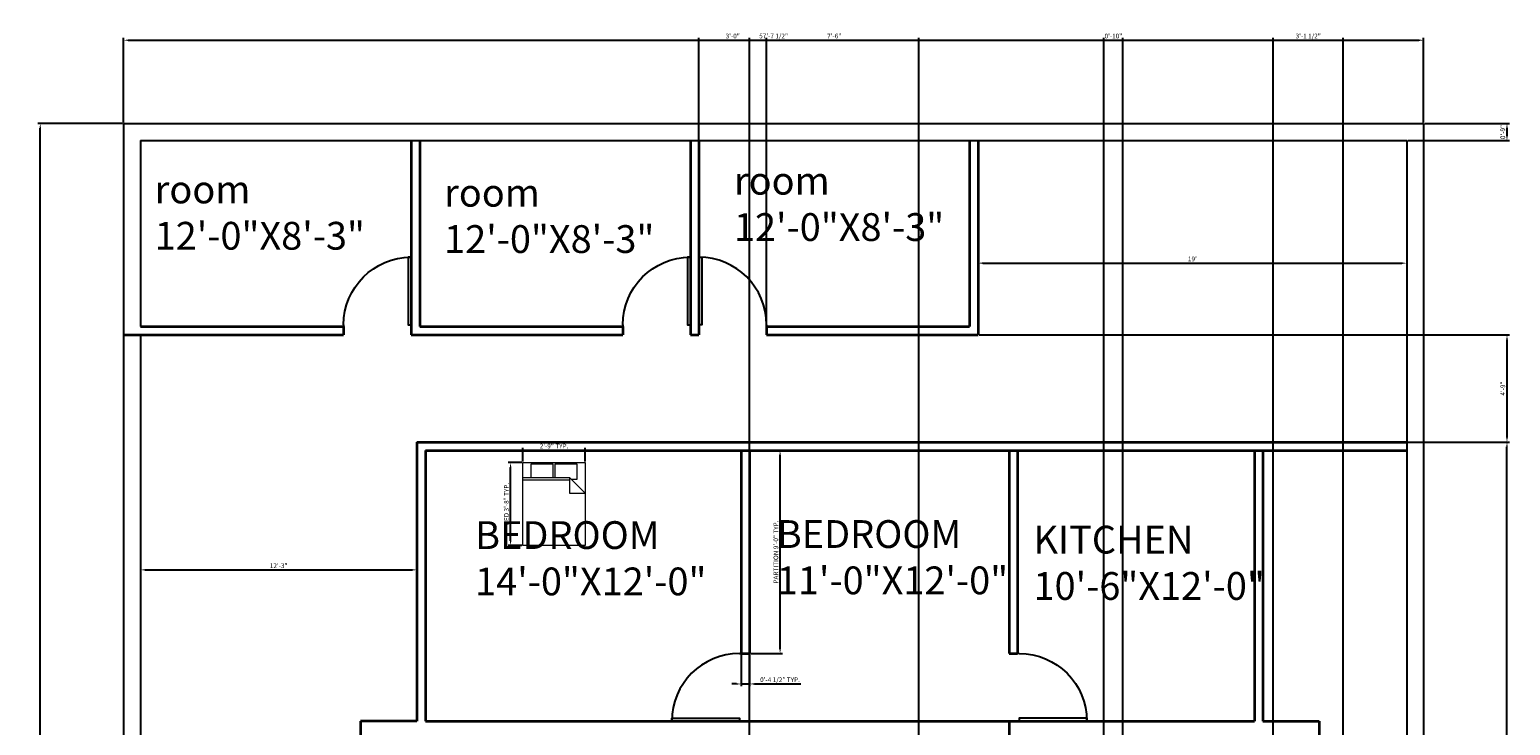
# Model space of a CAD drawing. Units: inches. Extents: x 357471052 to 714943146, y 500380981 to 1000762890.
# Tile 2 of 2: x 357471052 to 357471840, y 500381587 to 500381958. Entities that reach past the tile are written whole.
import ezdxf

# ---------------------------------------------------------------- set-up
doc = ezdxf.new("R2010")
doc.units = ezdxf.units.IN
for name, color, linetype, lineweight in [('A-ANNO-DIMS', 2, 'Continuous', 18), ('A-AREA-IDEN', 7, 'Continuous', 25), ('A-DOOR', 3, 'Continuous', 25), ('A-FURN', 9, 'Continuous', 18), ('A-WALL', 7, 'Continuous', 35), ('C-PROP', 8, 'Continuous', 25)]:
    doc.layers.add(name, color=color, linetype=linetype, lineweight=lineweight)
doc.styles.get("Standard").update_dxf_attribs({"font": 'arial.ttf'})
doc.dimstyles.new('ISO-25', dxfattribs={"dimtxt": 2.5, "dimasz": 2.5, "dimexe": 1.25, "dimexo": 0.625, "dimtad": 1, "dimlunit": 4, "dimtxsty": 'Standard', "dimcen": 2.5, "dimadec": 0, "dimazin": 0, "dimtfac": 1, "dimtmove": 0, "dimatfit": 3, "dimfxl": 1, "dimarcsym": 0})

# ---------------------------------------------------------------- blocks, each defined once
blk = doc.blocks.new('*U3')
for p, q in [((0, 0), (0, -6)), ((40, 0), (40, -6))]:
    blk.add_line(p, q)
blk.add_lwpolyline([(0, 0), (0, 40), (1.75, 40), (1.75, 0)], close=True)
blk.add_arc((0, 0), 40, 0, 90)
blk = doc.blocks.new('Bed - Queen')
for p, q in [((0, -80.00003), (0, 0)), ((0, 0), (59.99999, 0)), ((59.99999, 0), (59.99999, -80.00003)), ((7.99999, -1.2), (28.79998, -1.2)), ((7.99999, -14.4), (7.99999, -1.2)), ((28.79998, -1.2), (28.79998, -14.4)), ((31.19999, -1.2), (51.99999, -1.2)), ((31.19999, -14.4), (31.19999, -1.2)), ((51.99999, -1.2), (51.99999, -16.4)), ((0, -14.4), (44.8, -14.4)), ((44.8, -16.8), (0, -16.8)), ((59.99999, -29.6), (44.8, -14.4)), ((44.8, -14.4), (44.8, -29.6)), ((51.99999, -16.4), (46.79936, -16.4)), ((44.8, -29.6), (59.99999, -29.6)), ((59.99999, -80.00003), (0, -80.00003))]:
    blk.add_line(p, q)
blk = doc.blocks.new('*D5')
at = {"layer": 'A-ANNO-DIMS', "color": 0, "lineweight": -2, "transparency": 16777216}
for p, q in [((357471556.72, 500381848.42), (357471556.72, 500381832.02)), ((357471784.72, 500381848.42), (357471784.72, 500381832.02)), ((357471559.22, 500381833.27), (357471782.22, 500381833.27))]:
    blk.add_line(p, q, dxfattribs=at)
at = {"layer": 'A-ANNO-DIMS', "color": 0, "transparency": 16777216}
for points in [[(357471559.22, 500381833.68), (357471559.22, 500381832.85), (357471556.72, 500381833.27)], [(357471782.22, 500381833.68), (357471782.22, 500381832.85), (357471784.72, 500381833.27)]]:
    blk.add_solid(points, dxfattribs=at)
at = {"layer": 'Defpoints', "color": 0, "transparency": 16777216}
for p in [(357471556.72, 500381849.04), (357471784.72, 500381849.04), (357471784.72, 500381833.27)]:
    blk.add_point(p, dxfattribs=at)
at = {"layer": 'A-ANNO-DIMS', "color": 0, "transparency": 16777216, "insert": (357471670.72, 500381835.17), "char_height": 2.5, "attachment_point": 5}
blk.add_mtext("19'", dxfattribs=at)
blk = doc.blocks.new('*D6')
at = {"layer": 'A-ANNO-DIMS', "color": 0, "lineweight": -2, "transparency": 16777216}
for p, q in [((357471111.22, 500381678.37), (357471111.22, 500381668.81)), ((357471258.22, 500381678.37), (357471258.22, 500381668.81)), ((357471113.72, 500381670.06), (357471255.72, 500381670.06))]:
    blk.add_line(p, q, dxfattribs=at)
at = {"layer": 'A-ANNO-DIMS', "color": 0, "transparency": 16777216}
for points in [[(357471113.72, 500381670.48), (357471113.72, 500381669.64), (357471111.22, 500381670.06)], [(357471255.72, 500381670.48), (357471255.72, 500381669.64), (357471258.22, 500381670.06)]]:
    blk.add_solid(points, dxfattribs=at)
at = {"layer": 'Defpoints', "color": 0, "transparency": 16777216}
for p in [(357471111.22, 500381678.99), (357471258.22, 500381678.99), (357471258.22, 500381670.06)]:
    blk.add_point(p, dxfattribs=at)
at = {"layer": 'A-ANNO-DIMS', "color": 0, "transparency": 16777216, "insert": (357471184.72, 500381671.96), "char_height": 2.5, "attachment_point": 5}
blk.add_mtext('12\'-3"', dxfattribs=at)
blk = doc.blocks.new('PARTITION-108IN-CAPPED')
for p, q in [((0, 108), (0, 0)), ((4.5, 108), (4.5, 0)), ((0, 0), (4.5, 0))]:
    blk.add_line(p, q)
blk = doc.blocks.new('*D13')
at = {"layer": 'A-ANNO-DIMS', "color": 0, "lineweight": -2, "transparency": 16777216}
for p, q in [((357471314.03, 500381727.11), (357471306.8, 500381727.11)), ((357471308.05, 500381685.54), (357471308.05, 500381724.61)), ((357471314.03, 500381683.04), (357471306.8, 500381683.04))]:
    blk.add_line(p, q, dxfattribs=at)
at = {"layer": 'A-ANNO-DIMS', "color": 0, "transparency": 16777216}
for points in [[(357471307.63, 500381724.61), (357471308.47, 500381724.61), (357471308.05, 500381727.11)], [(357471307.63, 500381685.54), (357471308.47, 500381685.54), (357471308.05, 500381683.04)]]:
    blk.add_solid(points, dxfattribs=at)
at = {"layer": 'Defpoints', "color": 0, "transparency": 16777216}
for p in [(357471308.05, 500381727.11), (357471314.66, 500381727.11), (357471314.66, 500381683.04)]:
    blk.add_point(p, dxfattribs=at)
at = {"layer": 'A-ANNO-DIMS', "color": 0, "transparency": 16777216, "insert": (357471306.15, 500381705.08), "char_height": 2.5, "attachment_point": 5, "rotation": 90}
blk.add_mtext('BED 3\'-8" TYP.', dxfattribs=at)
blk = doc.blocks.new('*D14')
at = {"layer": 'A-ANNO-DIMS', "color": 0, "lineweight": -2, "transparency": 16777216}
for p, q in [((357471314.66, 500381727.73), (357471314.66, 500381734.97)), ((357471317.16, 500381733.72), (357471345.21, 500381733.72)), ((357471347.71, 500381727.73), (357471347.71, 500381734.97))]:
    blk.add_line(p, q, dxfattribs=at)
at = {"layer": 'A-ANNO-DIMS', "color": 0, "transparency": 16777216}
for points in [[(357471317.16, 500381734.13), (357471317.16, 500381733.3), (357471314.66, 500381733.72)], [(357471345.21, 500381734.13), (357471345.21, 500381733.3), (357471347.71, 500381733.72)]]:
    blk.add_solid(points, dxfattribs=at)
at = {"layer": 'Defpoints', "color": 0, "transparency": 16777216}
for p in [(357471347.71, 500381733.72), (357471314.66, 500381727.11), (357471347.71, 500381727.11)]:
    blk.add_point(p, dxfattribs=at)
at = {"layer": 'A-ANNO-DIMS', "color": 0, "transparency": 16777216, "insert": (357471331.18, 500381735.62), "char_height": 2.5, "attachment_point": 5}
blk.add_mtext('2\'-9" TYP.', dxfattribs=at)
blk = doc.blocks.new('*D15')
at = {"layer": 'A-ANNO-DIMS', "color": 0, "lineweight": -2, "transparency": 16777216}
for p, q in [((357471435.84, 500381733.54), (357471452.67, 500381733.54)), ((357471451.42, 500381628.04), (357471451.42, 500381731.04)), ((357471435.84, 500381625.54), (357471452.67, 500381625.54))]:
    blk.add_line(p, q, dxfattribs=at)
at = {"layer": 'A-ANNO-DIMS', "color": 0, "transparency": 16777216}
for points in [[(357471451, 500381731.04), (357471451.84, 500381731.04), (357471451.42, 500381733.54)], [(357471451, 500381628.04), (357471451.84, 500381628.04), (357471451.42, 500381625.54)]]:
    blk.add_solid(points, dxfattribs=at)
at = {"layer": 'Defpoints', "color": 0, "transparency": 16777216}
for p in [(357471435.22, 500381733.54), (357471451.42, 500381733.54), (357471435.22, 500381625.54)]:
    blk.add_point(p, dxfattribs=at)
at = {"layer": 'A-ANNO-DIMS', "color": 0, "transparency": 16777216, "insert": (357471449.5, 500381679.54), "char_height": 2.5, "attachment_point": 5, "rotation": 90}
blk.add_mtext('PARTITION 9\'-0" TYP.', dxfattribs=at)
blk = doc.blocks.new('*D16')
at = {"layer": 'A-ANNO-DIMS', "color": 0, "lineweight": -2, "transparency": 16777216}
for p, q in [((357471430.72, 500381624.92), (357471430.72, 500381608.09)), ((357471435.22, 500381624.92), (357471435.22, 500381608.09)), ((357471428.22, 500381609.34), (357471425.72, 500381609.34)), ((357471430.72, 500381609.34), (357471435.22, 500381609.34)), ((357471437.72, 500381609.34), (357471462.53, 500381609.34))]:
    blk.add_line(p, q, dxfattribs=at)
at = {"layer": 'A-ANNO-DIMS', "color": 0, "transparency": 16777216}
for points in [[(357471428.22, 500381609.76), (357471428.22, 500381608.93), (357471430.72, 500381609.34)], [(357471437.72, 500381609.76), (357471437.72, 500381608.93), (357471435.22, 500381609.34)]]:
    blk.add_solid(points, dxfattribs=at)
at = {"layer": 'Defpoints', "color": 0, "transparency": 16777216}
for p in [(357471430.72, 500381625.54), (357471435.22, 500381625.54), (357471435.22, 500381609.34)]:
    blk.add_point(p, dxfattribs=at)
at = {"layer": 'A-ANNO-DIMS', "color": 0, "transparency": 16777216, "insert": (357471451.38, 500381611.26), "char_height": 2.5, "attachment_point": 5}
blk.add_mtext('0\'-4 1/2" TYP.', dxfattribs=at)
blk = doc.blocks.new('*D21')
at = {"layer": 'A-ANNO-DIMS', "color": 0, "lineweight": -2, "transparency": 16777216}
for p, q in [((357471102.22, 500381908.17), (357471102.22, 500381953.14)), ((357471104.72, 500381951.89), (357471791.22, 500381951.89)), ((357471793.72, 500381908.17), (357471793.72, 500381953.14))]:
    blk.add_line(p, q, dxfattribs=at)
at = {"layer": 'A-ANNO-DIMS', "color": 0, "transparency": 16777216}
for points in [[(357471104.72, 500381952.31), (357471104.72, 500381951.48), (357471102.22, 500381951.89)], [(357471791.22, 500381952.31), (357471791.22, 500381951.48), (357471793.72, 500381951.89)]]:
    blk.add_solid(points, dxfattribs=at)
at = {"layer": 'Defpoints', "color": 0, "transparency": 16777216}
for p in [(357471793.72, 500381951.89), (357471102.22, 500381907.54), (357471793.72, 500381907.54)]:
    blk.add_point(p, dxfattribs=at)
at = {"layer": 'A-ANNO-DIMS', "color": 0, "transparency": 16777216, "insert": (357471447.97, 500381953.81), "char_height": 2.5, "attachment_point": 5}
blk.add_mtext('57\'-7 1/2"', dxfattribs=at)
blk = doc.blocks.new('*D22')
at = {"layer": 'A-ANNO-DIMS', "color": 0, "lineweight": -2, "transparency": 16777216}
for p, q in [((357471101.59, 500381907.54), (357471056.62, 500381907.54)), ((357471057.87, 500381029.54), (357471057.87, 500381905.04)), ((357471101.59, 500381027.04), (357471056.62, 500381027.04))]:
    blk.add_line(p, q, dxfattribs=at)
at = {"layer": 'A-ANNO-DIMS', "color": 0, "transparency": 16777216}
for points in [[(357471057.45, 500381905.04), (357471058.29, 500381905.04), (357471057.87, 500381907.54)], [(357471057.45, 500381029.54), (357471058.29, 500381029.54), (357471057.87, 500381027.04)]]:
    blk.add_solid(points, dxfattribs=at)
at = {"layer": 'Defpoints', "color": 0, "transparency": 16777216}
for p in [(357471057.87, 500381907.54), (357471102.22, 500381907.54), (357471102.22, 500381027.04)]:
    blk.add_point(p, dxfattribs=at)
at = {"layer": 'A-ANNO-DIMS', "color": 0, "transparency": 16777216, "insert": (357471055.95, 500381467.29), "char_height": 2.5, "attachment_point": 5, "rotation": 90}
blk.add_mtext('73\'-4 1/2"', dxfattribs=at)
blk = doc.blocks.new('*D24')
at = {"layer": 'A-ANNO-DIMS', "color": 0, "lineweight": -2, "transparency": 16777216}
for p, q in [((357471785.34, 500381738.04), (357471839.32, 500381738.04)), ((357471838.07, 500381103.04), (357471838.07, 500381735.54)), ((357471561.84, 500381100.54), (357471839.32, 500381100.54))]:
    blk.add_line(p, q, dxfattribs=at)
at = {"layer": 'A-ANNO-DIMS', "color": 0, "transparency": 16777216}
for points in [[(357471837.65, 500381735.54), (357471838.49, 500381735.54), (357471838.07, 500381738.04)], [(357471837.65, 500381103.04), (357471838.49, 500381103.04), (357471838.07, 500381100.54)]]:
    blk.add_solid(points, dxfattribs=at)
at = {"layer": 'Defpoints', "color": 0, "transparency": 16777216}
for p in [(357471784.72, 500381738.04), (357471838.07, 500381738.04), (357471561.22, 500381100.54)]:
    blk.add_point(p, dxfattribs=at)
at = {"layer": 'A-ANNO-DIMS', "color": 0, "transparency": 16777216, "insert": (357471836.15, 500381419.29), "char_height": 2.5, "attachment_point": 5, "rotation": 90}
blk.add_mtext('53\'-1 1/2"', dxfattribs=at)
blk = doc.blocks.new('*D25')
at = {"layer": 'A-ANNO-DIMS', "color": 0, "lineweight": -2, "transparency": 16777216}
for p, q in [((357471557.34, 500381795.04), (357471839.32, 500381795.04)), ((357471838.07, 500381792.54), (357471838.07, 500381740.54)), ((357471785.34, 500381738.04), (357471839.32, 500381738.04))]:
    blk.add_line(p, q, dxfattribs=at)
at = {"layer": 'A-ANNO-DIMS', "color": 0, "transparency": 16777216}
for points in [[(357471837.65, 500381792.54), (357471838.49, 500381792.54), (357471838.07, 500381795.04)], [(357471837.65, 500381740.54), (357471838.49, 500381740.54), (357471838.07, 500381738.04)]]:
    blk.add_solid(points, dxfattribs=at)
at = {"layer": 'Defpoints', "color": 0, "transparency": 16777216}
for p in [(357471556.72, 500381795.04), (357471784.72, 500381738.04), (357471838.07, 500381738.04)]:
    blk.add_point(p, dxfattribs=at)
at = {"layer": 'A-ANNO-DIMS', "color": 0, "transparency": 16777216, "insert": (357471836.17, 500381766.54), "char_height": 2.5, "attachment_point": 5, "rotation": 90}
blk.add_mtext('4\'-9"', dxfattribs=at)
blk = doc.blocks.new('*D26')
at = {"layer": 'A-ANNO-DIMS', "color": 0, "lineweight": -2, "transparency": 16777216}
for p, q in [((357471408.22, 500381795.67), (357471408.22, 500381953.14)), ((357471410.72, 500381951.89), (357471441.72, 500381951.89)), ((357471444.22, 500381795.67), (357471444.22, 500381953.14))]:
    blk.add_line(p, q, dxfattribs=at)
at = {"layer": 'A-ANNO-DIMS', "color": 0, "transparency": 16777216}
for points in [[(357471410.72, 500381952.31), (357471410.72, 500381951.48), (357471408.22, 500381951.89)], [(357471441.72, 500381952.31), (357471441.72, 500381951.48), (357471444.22, 500381951.89)]]:
    blk.add_solid(points, dxfattribs=at)
at = {"layer": 'Defpoints', "color": 0, "transparency": 16777216}
for p in [(357471444.22, 500381951.89), (357471408.22, 500381795.04), (357471444.22, 500381795.04)]:
    blk.add_point(p, dxfattribs=at)
at = {"layer": 'A-ANNO-DIMS', "color": 0, "transparency": 16777216, "insert": (357471426.22, 500381953.8), "char_height": 2.5, "attachment_point": 5}
blk.add_mtext('3\'-0"', dxfattribs=at)
blk = doc.blocks.new('*D29')
at = {"layer": 'A-ANNO-DIMS', "color": 0, "lineweight": -2, "transparency": 16777216}
for p, q in [((357471794.34, 500381907.54), (357471839.32, 500381907.54)), ((357471838.07, 500381905.04), (357471838.07, 500381901.04)), ((357471785.34, 500381898.54), (357471839.32, 500381898.54))]:
    blk.add_line(p, q, dxfattribs=at)
at = {"layer": 'A-ANNO-DIMS', "color": 0, "transparency": 16777216}
for points in [[(357471837.65, 500381905.04), (357471838.49, 500381905.04), (357471838.07, 500381907.54)], [(357471837.65, 500381901.04), (357471838.49, 500381901.04), (357471838.07, 500381898.54)]]:
    blk.add_solid(points, dxfattribs=at)
at = {"layer": 'Defpoints', "color": 0, "transparency": 16777216}
for p in [(357471793.72, 500381907.54), (357471784.72, 500381898.54), (357471838.07, 500381898.54)]:
    blk.add_point(p, dxfattribs=at)
at = {"layer": 'A-ANNO-DIMS', "color": 0, "transparency": 16777216, "insert": (357471836.17, 500381903.04), "char_height": 2.5, "attachment_point": 5, "rotation": 90}
blk.add_mtext('0\'-9"', dxfattribs=at)
blk = doc.blocks.new('*D30')
at = {"layer": 'A-ANNO-DIMS', "color": 0, "lineweight": -2, "transparency": 16777216}
for p, q in [((357471435.22, 500381149.17), (357471435.22, 500381953.14)), ((357471437.72, 500381951.89), (357471522.72, 500381951.89)), ((357471525.22, 500381149.17), (357471525.22, 500381953.14))]:
    blk.add_line(p, q, dxfattribs=at)
at = {"layer": 'A-ANNO-DIMS', "color": 0, "transparency": 16777216}
for points in [[(357471437.72, 500381952.31), (357471437.72, 500381951.48), (357471435.22, 500381951.89)], [(357471522.72, 500381952.31), (357471522.72, 500381951.48), (357471525.22, 500381951.89)]]:
    blk.add_solid(points, dxfattribs=at)
at = {"layer": 'Defpoints', "color": 0, "transparency": 16777216}
for p in [(357471525.22, 500381951.89), (357471435.22, 500381148.54), (357471525.22, 500381148.54)]:
    blk.add_point(p, dxfattribs=at)
at = {"layer": 'A-ANNO-DIMS', "color": 0, "transparency": 16777216, "insert": (357471480.22, 500381953.79), "char_height": 2.5, "attachment_point": 5}
blk.add_mtext('7\'-6"', dxfattribs=at)
blk = doc.blocks.new('*D31')
at = {"layer": 'A-ANNO-DIMS', "color": 0, "lineweight": -2, "transparency": 16777216}
for p, q in [((357471623.71, 500381374.17), (357471623.71, 500381953.14)), ((357471626.21, 500381951.89), (357471631.21, 500381951.89)), ((357471633.71, 500381374.24), (357471633.71, 500381953.14))]:
    blk.add_line(p, q, dxfattribs=at)
at = {"layer": 'A-ANNO-DIMS', "color": 0, "transparency": 16777216}
for points in [[(357471626.21, 500381952.31), (357471626.21, 500381951.48), (357471623.71, 500381951.89)], [(357471631.21, 500381952.31), (357471631.21, 500381951.48), (357471633.71, 500381951.89)]]:
    blk.add_solid(points, dxfattribs=at)
at = {"layer": 'Defpoints', "color": 0, "transparency": 16777216}
for p in [(357471633.71, 500381951.89), (357471623.71, 500381373.54), (357471633.71, 500381373.61)]:
    blk.add_point(p, dxfattribs=at)
at = {"layer": 'A-ANNO-DIMS', "color": 0, "transparency": 16777216, "insert": (357471628.71, 500381953.79), "char_height": 2.5, "attachment_point": 5}
blk.add_mtext('0\'-10"', dxfattribs=at)
blk = doc.blocks.new('*D32')
at = {"layer": 'A-ANNO-DIMS', "color": 0, "lineweight": -2, "transparency": 16777216}
for p, q in [((357471713.71, 500381443.46), (357471713.71, 500381953.14)), ((357471716.21, 500381951.89), (357471748.47, 500381951.89)), ((357471750.97, 500381443.17), (357471750.97, 500381953.14))]:
    blk.add_line(p, q, dxfattribs=at)
at = {"layer": 'A-ANNO-DIMS', "color": 0, "transparency": 16777216}
for points in [[(357471716.21, 500381952.31), (357471716.21, 500381951.48), (357471713.71, 500381951.89)], [(357471748.47, 500381952.31), (357471748.47, 500381951.48), (357471750.97, 500381951.89)]]:
    blk.add_solid(points, dxfattribs=at)
at = {"layer": 'Defpoints', "color": 0, "transparency": 16777216}
for p in [(357471750.97, 500381951.89), (357471713.71, 500381442.83), (357471750.97, 500381442.54)]:
    blk.add_point(p, dxfattribs=at)
at = {"layer": 'A-ANNO-DIMS', "color": 0, "transparency": 16777216, "insert": (357471732.34, 500381953.81), "char_height": 2.5, "attachment_point": 5}
blk.add_mtext('3\'-1 1/2"', dxfattribs=at)

msp = doc.modelspace()

# ---------------------------------------------------------------- linework, layer by layer
at = {"layer": 'A-WALL'}
for p, q in [((357471255.219, 500381898.543), (357471255.219, 500381795.043)), ((357471259.719, 500381898.543), (357471259.719, 500381799.543)), ((357471403.719, 500381898.543), (357471403.719, 500381795.043)), ((357471408.219, 500381898.543), (357471408.219, 500381795.043)), ((357471552.219, 500381898.543), (357471552.219, 500381799.543)), ((357471556.719, 500381898.543), (357471556.719, 500381795.043)), ((357471556.719, 500381898.543), (357471556.719, 500381799.543)), ((357471111.219, 500381799.543), (357471219.219, 500381799.543)), ((357471219.219, 500381799.543), (357471219.219, 500381795.043)), ((357471259.719, 500381799.543), (357471367.719, 500381799.543)), ((357471367.719, 500381799.543), (357471367.719, 500381795.043)), ((357471444.219, 500381799.543), (357471552.219, 500381799.543)), ((357471444.219, 500381799.543), (357471444.219, 500381795.043)), ((357471102.219, 500381795.043), (357471219.219, 500381795.043)), ((357471255.219, 500381795.043), (357471367.719, 500381795.043)), ((357471403.719, 500381795.043), (357471408.219, 500381795.043)), ((357471444.219, 500381795.043), (357471556.719, 500381795.043)), ((357471258.219, 500381738.043), (357471784.719, 500381738.043)), ((357471258.219, 500381738.043), (357471258.219, 500381589.543)), ((357471262.719, 500381733.543), (357471784.719, 500381733.543)), ((357471262.719, 500381733.543), (357471262.719, 500381589.543)), ((357471703.719, 500381733.543), (357471703.719, 500381589.543)), ((357471708.219, 500381733.543), (357471708.219, 500381589.543)), ((357471258.219, 500381589.543), (357471228.219, 500381589.543)), ((357471228.219, 500381589.543), (357471228.219, 500381442.543)), ((357471262.719, 500381589.543), (357471703.719, 500381589.543)), ((357471573.219, 500381589.543), (357471573.219, 500381325.543)), ((357471708.219, 500381589.543), (357471738.219, 500381589.543)), ((357471738.219, 500381589.543), (357471738.219, 500381442.543))]:
    msp.add_line(p, q, dxfattribs=at)
at = {"layer": 'C-PROP'}
for p, q in [((357471102.219, 500381907.543), (357471102.219, 500381027.043)), ((357471102.219, 500381907.543), (357471793.719, 500381907.543)), ((357471793.719, 500381907.543), (357471793.719, 500381795.043)), ((357471111.219, 500381898.543), (357471784.719, 500381898.543)), ((357471111.219, 500381898.543), (357471111.219, 500381799.543)), ((357471784.719, 500381898.543), (357471784.719, 500381795.043)), ((357471111.219, 500381795.043), (357471111.219, 500381027.043)), ((357471784.719, 500381795.043), (357471784.719, 500381027.043)), ((357471793.719, 500381795.043), (357471793.719, 500381027.043))]:
    msp.add_line(p, q, dxfattribs=at)

# ---------------------------------------------------------------- block references
at = {"layer": 'A-DOOR', "yscale": 0.9, "zscale": 0.9}
for p, xscale in [((357471255.219, 500381800.443), -0.9), ((357471403.719, 500381800.443), -0.9), ((357471408.219, 500381800.443), 0.9)]:
    msp.add_blockref('*U3', p, dxfattribs=dict(at, xscale=xscale))
for p, xscale, rotation in [((357471429.819, 500381589.543), 0.9, 90), ((357471578.619, 500381589.543), -0.9, 270)]:
    msp.add_blockref('*U3', p, dxfattribs=dict(at, xscale=xscale, rotation=rotation))
at = {"layer": 'A-FURN', "xscale": 0.5508172427300339, "yscale": 0.5508172427300339, "zscale": 0.5508172427300339}
msp.add_blockref('Bed - Queen', (357471314.659, 500381727.108), dxfattribs=at)
at = {"layer": 'A-WALL'}
for p in [(357471430.719, 500381625.543), (357471573.219, 500381625.543)]:
    msp.add_blockref('PARTITION-108IN-CAPPED', p, dxfattribs=at)

# ---------------------------------------------------------------- texts
at = {"layer": 'A-AREA-IDEN', "char_height": 14.78481, "attachment_point": 1}
for s, insert in [('room\\P12\'-0"X8\'-3"', (357471118.729, 500381879.872)), ('room\\P12\'-0"X8\'-3"', (357471426.87, 500381884.505)), ('room\\P12\'-0"X8\'-3"', (357471272.702, 500381878.123)), ('BEDROOM\\P14\'-0"X12\'-0"', (357471289.195, 500381695.945)), ('BEDROOM\\P11\'-0"X12\'-0"', (357471449.678, 500381696.503)), ('KITCHEN\\P10\'-6"X12\'-0"', (357471586.216, 500381693.521))]:
    msp.add_mtext_dynamic_manual_height_columns(s, width=42.9623, gutter_width=73.924, heights=[0], dxfattribs=dict(at, insert=insert))

# ---------------------------------------------------------------- dimensions: what is measured, and where the dimension line sits
at = {"layer": 'A-ANNO-DIMS'}
for base, p1, p2, override, picture, middle in [((357471793.719, 500381951.893), (357471102.219, 500381907.543), (357471793.719, 500381907.543), {"dimdec": 1, "dimlfac": 1, "dimrnd": 0, "dimzin": 1, "dimdsep": 46, "dimlunit": 4, "dimfrac": 2}, '*D21', (357471447.969, 500381953.81)), ((357471444.219, 500381951.893), (357471408.219, 500381795.043), (357471444.219, 500381795.043), {"dimdec": 1, "dimlfac": 1, "dimrnd": 0, "dimzin": 1, "dimdsep": 46, "dimlunit": 4, "dimfrac": 2}, '*D26', (357471426.219, 500381953.795)), ((357471525.219, 500381951.893), (357471435.219, 500381148.543), (357471525.219, 500381148.543), {"dimdec": 1, "dimlfac": 1, "dimrnd": 0, "dimzin": 1, "dimdsep": 46, "dimlunit": 4, "dimfrac": 2}, '*D30', (357471480.219, 500381953.794)), ((357471633.713, 500381951.893), (357471623.714, 500381373.543), (357471633.713, 500381373.612), {"dimdec": 1, "dimlfac": 1, "dimrnd": 0, "dimzin": 1, "dimdsep": 46, "dimlunit": 4, "dimfrac": 2}, '*D31', (357471628.713, 500381953.794)), ((357471750.974, 500381951.893), (357471713.711, 500381442.834), (357471750.974, 500381442.543), {"dimdec": 1, "dimlfac": 1, "dimrnd": 0, "dimzin": 1, "dimdsep": 46, "dimlunit": 4, "dimfrac": 2}, '*D32', (357471732.343, 500381953.811)), ((357471784.719, 500381833.268), (357471556.719, 500381849.043), (357471784.719, 500381849.043), {"dimclrd": 0, "dimclre": 0, "dimclrt": 0}, '*D5', (357471670.719, 500381835.17)), ((357471258.219, 500381670.059), (357471111.219, 500381678.993), (357471258.219, 500381678.993), {"dimclrd": 0, "dimclre": 0, "dimclrt": 0}, '*D6', (357471184.719, 500381671.962))]:
    dim = msp.add_linear_dim(base=base, p1=p1, p2=p2, dimstyle='ISO-25', override=override, dxfattribs=at)
    dim.commit()
    dim.dimension.update_dxf_attribs({"geometry": picture, "text_midpoint": middle})
for base, p1, p2, picture, middle in [((357471057.869, 500381907.543), (357471102.219, 500381027.043), (357471102.219, 500381907.543), '*D22', (357471055.951, 500381467.293)), ((357471838.069, 500381898.543), (357471793.719, 500381907.543), (357471784.719, 500381898.543), '*D29', (357471836.168, 500381903.043)), ((357471838.069, 500381738.043), (357471556.719, 500381795.043), (357471784.719, 500381738.043), '*D25', (357471836.168, 500381766.543)), ((357471838.069, 500381738.043), (357471561.219, 500381100.543), (357471784.719, 500381738.043), '*D24', (357471836.151, 500381419.293))]:
    dim = msp.add_linear_dim(base=base, p1=p1, p2=p2, angle=90, dimstyle='ISO-25', override={"dimdec": 1, "dimlfac": 1, "dimrnd": 0, "dimzin": 1, "dimdsep": 46, "dimlunit": 4, "dimfrac": 2}, dxfattribs=at)
    dim.commit()
    dim.dimension.update_dxf_attribs({"geometry": picture, "text_midpoint": middle})
for base, p1, p2, picture, middle in [((357471347.708, 500381733.718), (357471314.659, 500381727.108), (357471347.708, 500381727.108), '*D14', (357471331.183, 500381735.619)), ((357471435.219, 500381609.343), (357471430.719, 500381625.543), (357471435.219, 500381625.543), '*D16', (357471451.376, 500381611.26))]:
    dim = msp.add_linear_dim(base=base, p1=p1, p2=p2, text='<> TYP.', dimstyle='ISO-25', override={"dimdec": 1, "dimlfac": 1, "dimrnd": 0, "dimzin": 1, "dimdsep": 46, "dimlunit": 4, "dimfrac": 2}, dxfattribs=at)
    dim.commit()
    dim.dimension.update_dxf_attribs({"geometry": picture, "text_midpoint": middle})
for base, p1, p2, text, picture, middle in [((357471451.419, 500381733.543), (357471435.219, 500381625.543), (357471435.219, 500381733.543), 'PARTITION <> TYP.', '*D15', (357471449.501, 500381679.543)), ((357471308.049, 500381727.108), (357471314.659, 500381683.042), (357471314.659, 500381727.108), 'BED <> TYP.', '*D13', (357471306.147, 500381705.075))]:
    dim = msp.add_linear_dim(base=base, p1=p1, p2=p2, angle=90, text=text, dimstyle='ISO-25', override={"dimdec": 1, "dimlfac": 1, "dimrnd": 0, "dimzin": 1, "dimdsep": 46, "dimlunit": 4, "dimfrac": 2}, dxfattribs=at)
    dim.commit()
    dim.dimension.update_dxf_attribs({"geometry": picture, "text_midpoint": middle})

doc.saveas('drawing.dxf')
